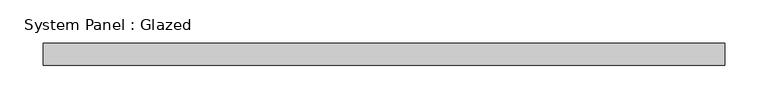
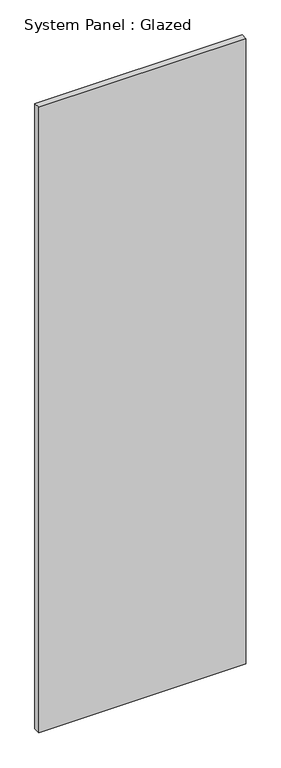
"""IFC4 building model written with IfcOpenShell, lengths in millimetres: plate geometry, System Panel : Glazed."""

from ifc_helpers import new_model, si_unit, origin, origin_with_axes, place, context, project, spatial, polyline, outline, extrude, source, transform, mapped, element, save


def system_panel_glazed_923938e8(model_context):
    return source(origin(), model_context, "Body", "SweptSolid", [
        extrude(outline(polyline([(393.7, 19.05), (-393.7, 19.05), (-393.7, 44.45), (393.7, 44.45), (393.7, 19.05)])), origin_with_axes(), (0.0, 0.0, 1.0), 2514.6),
    ])


if __name__ == "__main__":
    model = new_model("IFC4")
    model_context = context("Model", 3, world=origin())
    ifc_project = project(units=[si_unit("LENGTHUNIT", "METRE", prefix="MILLI")], contexts=[model_context])
    site = spatial("IfcSite", under=ifc_project)
    building = spatial("IfcBuilding", under=site)
    placement = place(None, origin())
    system_panel_glazed_shape = system_panel_glazed_923938e8(model_context)
    element("IfcPlate", 1, ObjectType="System Panel : Glazed", at=placement, inside=building, context=model_context, shape_type="MappedRepresentation", body=[
        mapped(system_panel_glazed_shape, transform((0.0, 0.0, 0.0), x_axis=(1.0, 0.0, 0.0), y_axis=(0.0, 1.0, 0.0), z_axis=(0.0, 0.0, 1.0))),
    ])
    save(model, "model.ifc")

# Revit data of these elements
# Type "System Panel : Glazed"
#   Construction Type Id = "GSP4R"
#   Analytic Construction = "1/8 in Pilkington single glazing"
#   Visual Light Transmittance = 0.9
#   Solar Heat Gain Coefficient = 0.86
#   Heat Transfer Coefficient (U) = 1.18115 BTU/(h·ft²·°F)
#   Define Thermal Properties by = 1
# Element 1 (IfcPlate, "System Panel : Glazed")
#   Materials on its faces: "Glass"
# Materials
#   "Glass": class "Glass", colour RGB 0 128 192, transparency 0.75, Description = "Soda Lime Glass", Cost = 0
